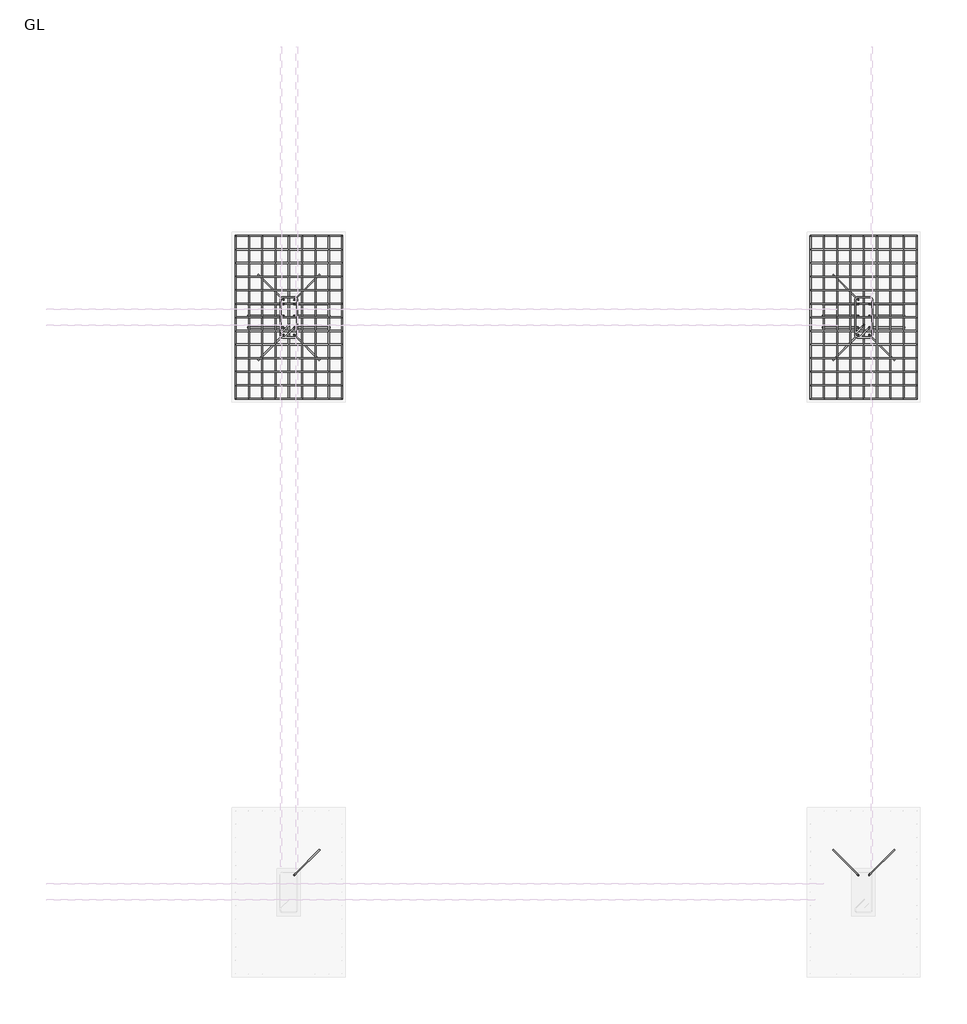
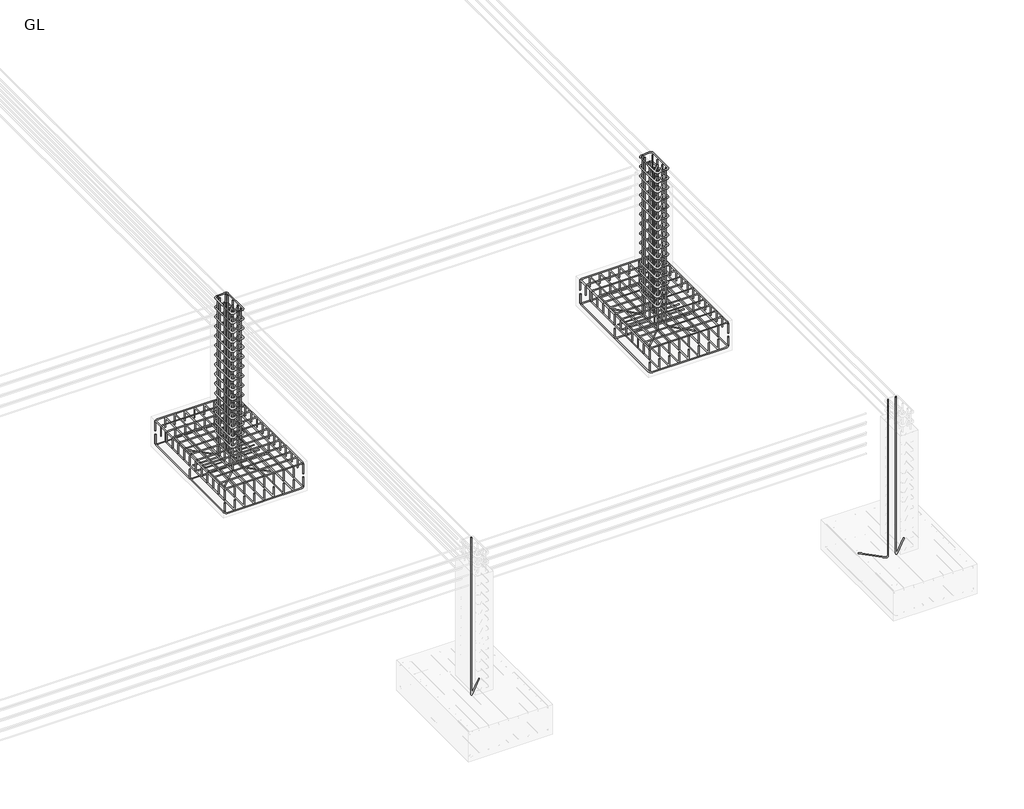
# One storey, part 11 of 16: 24 reinforcing bars.
"""IFC4 building model written with IfcOpenShell, lengths in millimetres."""

from ifc_helpers import new_model, si_unit, point, frame, origin, place, context, project, spatial, polyline, circle_curve, trimmed, segment, composite_curve, source, transform, mapped, element, save
from ifc_brep_helpers import swept_disk

model = new_model("IFC4")

# Units and contexts
model_context = context("Model", 3, world=origin())
ifc_project = project(units=[si_unit("LENGTHUNIT", "METRE", prefix="MILLI")], contexts=[model_context])

# Site, building, storey
site = spatial("IfcSite", under=ifc_project)
building = spatial("IfcBuilding", under=site)
storey = spatial("IfcBuildingStorey", under=building, Name="GL", Elevation=-1829.0)

# Reinforcing bars
placement = place(None, origin())
reinforcing_bar_shape = source(origin(), model_context, "Body", "SolidModel", [
    swept_disk(composite_curve([segment(polyline([(8237.0455621, -13319.1167521, -2089.0), (8237.0455621, -13319.1167521, -2213.0)]), True, "CONTINUOUS"), segment(trimmed(circle_curve(frame((8207.0455621, -13319.1167521, -2213.0), z_axis=(0.0, 1.0, 0.0), x_axis=(30.0, 0.0, 0.0)), 30.0), [point((8237.0455621, -13319.1167521, -2213.0))], [point((8207.0455621, -13319.1167521, -2243.0))], True, "CARTESIAN"), True, "CONTINUOUS"), segment(polyline([(8207.0455621, -13319.1167521, -2243.0), (7139.0455621, -13319.1167521, -2243.0)]), True, "CONTINUOUS"), segment(trimmed(circle_curve(frame((7139.0455621, -13319.1167521, -2213.0), z_axis=(0.0, 1.0, 0.0), x_axis=(0.0, 0.0, -30.0)), 30.0), [point((7139.0455621, -13319.1167521, -2243.0))], [point((7109.0455621, -13319.1167521, -2213.0))], True, "CARTESIAN"), True, "CONTINUOUS"), segment(polyline([(7109.0455621, -13319.1167521, -2213.0), (7109.0455621, -13319.1167521, -2089.0)]), True, "CONTINUOUS")], self_intersect=False), 6.0),
])
element("IfcReinforcingBar", 1, at=placement, inside=storey, context=model_context, shape_type="MappedRepresentation", body=[
    mapped(reinforcing_bar_shape, transform((0.0, 0.0, 0.0), x_axis=(1.0, 0.0, 0.0), y_axis=(0.0, 1.0, 0.0), z_axis=(0.0, 0.0, 1.0))),
    mapped(reinforcing_bar_shape, transform((0.0, -864.0, 0.0), x_axis=(1.0, 0.0, 0.0), y_axis=(0.0, 1.0, 0.0), z_axis=(0.0, 0.0, 1.0))),
    mapped(reinforcing_bar_shape, transform((0.0, -1728.0, 0.0), x_axis=(1.0, 0.0, 0.0), y_axis=(0.0, 1.0, 0.0), z_axis=(0.0, 0.0, 1.0))),
])
reinforcing_bar_2_shape = source(origin(), model_context, "Body", "SolidModel", [
    swept_disk(composite_curve([segment(polyline([(7109.0455621, -13319.1167521, -2022.436678), (7109.0455621, -13319.1167521, -1898.436678)]), True, "CONTINUOUS"), segment(trimmed(circle_curve(frame((7139.0455621, -13319.1167521, -1898.436678), z_axis=(0.0, 1.0, 0.0), x_axis=(-30.0, 0.0, 0.0)), 30.0), [point((7109.0455621, -13319.1167521, -1898.436678))], [point((7139.0455621, -13319.1167521, -1868.436678))], True, "CARTESIAN"), True, "CONTINUOUS"), segment(polyline([(7139.0455621, -13319.1167521, -1868.436678), (8207.0455621, -13319.1167521, -1868.436678)]), True, "CONTINUOUS"), segment(trimmed(circle_curve(frame((8207.0455621, -13319.1167521, -1898.436678), z_axis=(0.0, 1.0, 0.0), x_axis=(0.0, 0.0, 30.0)), 30.0), [point((8207.0455621, -13319.1167521, -1868.436678))], [point((8237.0455621, -13319.1167521, -1898.436678))], True, "CARTESIAN"), True, "CONTINUOUS"), segment(polyline([(8237.0455621, -13319.1167521, -1898.436678), (8237.0455621, -13319.1167521, -2022.436678)]), True, "CONTINUOUS")], self_intersect=False), 6.0),
])
element("IfcReinforcingBar", 2, at=placement, inside=storey, context=model_context, shape_type="MappedRepresentation", body=[
    mapped(reinforcing_bar_2_shape, transform((0.0, 0.0, 0.0), x_axis=(1.0, 0.0, 0.0), y_axis=(0.0, 1.0, 0.0), z_axis=(0.0, 0.0, 1.0))),
    mapped(reinforcing_bar_2_shape, transform((0.0, -144.0, 0.0), x_axis=(1.0, 0.0, 0.0), y_axis=(0.0, 1.0, 0.0), z_axis=(0.0, 0.0, 1.0))),
    mapped(reinforcing_bar_2_shape, transform((0.0, -288.0, 0.0), x_axis=(1.0, 0.0, 0.0), y_axis=(0.0, 1.0, 0.0), z_axis=(0.0, 0.0, 1.0))),
    mapped(reinforcing_bar_2_shape, transform((0.0, -432.0, 0.0), x_axis=(1.0, 0.0, 0.0), y_axis=(0.0, 1.0, 0.0), z_axis=(0.0, 0.0, 1.0))),
    mapped(reinforcing_bar_2_shape, transform((0.0, -576.0, 0.0), x_axis=(1.0, 0.0, 0.0), y_axis=(0.0, 1.0, 0.0), z_axis=(0.0, 0.0, 1.0))),
    mapped(reinforcing_bar_2_shape, transform((0.0, -720.0, 0.0), x_axis=(1.0, 0.0, 0.0), y_axis=(0.0, 1.0, 0.0), z_axis=(0.0, 0.0, 1.0))),
    mapped(reinforcing_bar_2_shape, transform((0.0, -864.0, 0.0), x_axis=(1.0, 0.0, 0.0), y_axis=(0.0, 1.0, 0.0), z_axis=(0.0, 0.0, 1.0))),
    mapped(reinforcing_bar_2_shape, transform((0.0, -1008.0, 0.0), x_axis=(1.0, 0.0, 0.0), y_axis=(0.0, 1.0, 0.0), z_axis=(0.0, 0.0, 1.0))),
    mapped(reinforcing_bar_2_shape, transform((0.0, -1152.0, 0.0), x_axis=(1.0, 0.0, 0.0), y_axis=(0.0, 1.0, 0.0), z_axis=(0.0, 0.0, 1.0))),
    mapped(reinforcing_bar_2_shape, transform((0.0, -1296.0, 0.0), x_axis=(1.0, 0.0, 0.0), y_axis=(0.0, 1.0, 0.0), z_axis=(0.0, 0.0, 1.0))),
    mapped(reinforcing_bar_2_shape, transform((0.0, -1440.0, 0.0), x_axis=(1.0, 0.0, 0.0), y_axis=(0.0, 1.0, 0.0), z_axis=(0.0, 0.0, 1.0))),
    mapped(reinforcing_bar_2_shape, transform((0.0, -1584.0, 0.0), x_axis=(1.0, 0.0, 0.0), y_axis=(0.0, 1.0, 0.0), z_axis=(0.0, 0.0, 1.0))),
    mapped(reinforcing_bar_2_shape, transform((0.0, -1728.0, 0.0), x_axis=(1.0, 0.0, 0.0), y_axis=(0.0, 1.0, 0.0), z_axis=(0.0, 0.0, 1.0))),
])
reinforcing_bar_3_shape = source(origin(), model_context, "Body", "SolidModel", [
    swept_disk(composite_curve([segment(polyline([(7109.0455621, -15047.1167521, -2027.5081232), (7109.0455621, -15047.1167521, -1903.5081232)]), True, "CONTINUOUS"), segment(trimmed(circle_curve(frame((7109.0455621, -15017.1167521, -1903.5081232), z_axis=(-1.0, 0.0, 0.0), x_axis=(0.0, -30.0, 0.0)), 30.0), [point((7109.0455621, -15047.1167521, -1903.5081232))], [point((7109.0455621, -15017.1167521, -1873.5081232))], True, "CARTESIAN"), True, "CONTINUOUS"), segment(polyline([(7109.0455621, -15017.1167521, -1873.5081232), (7109.0455621, -13349.1167521, -1873.5081232)]), True, "CONTINUOUS"), segment(trimmed(circle_curve(frame((7109.0455621, -13349.1167521, -1903.5081232), z_axis=(-1.0, 0.0, 0.0), x_axis=(0.0, 0.0, 30.0)), 30.0), [point((7109.0455621, -13349.1167521, -1873.5081232))], [point((7109.0455621, -13319.1167521, -1903.5081232))], True, "CARTESIAN"), True, "CONTINUOUS"), segment(polyline([(7109.0455621, -13319.1167521, -1903.5081232), (7109.0455621, -13319.1167521, -2027.5081232)]), True, "CONTINUOUS")], self_intersect=False), 6.0),
])
element("IfcReinforcingBar", 3, at=placement, inside=storey, context=model_context, shape_type="MappedRepresentation", body=[
    mapped(reinforcing_bar_3_shape, transform((0.0, 0.0, 0.0), x_axis=(1.0, 0.0, 0.0), y_axis=(0.0, 1.0, 0.0), z_axis=(0.0, 0.0, 1.0))),
    mapped(reinforcing_bar_3_shape, transform((141.0, 0.0, 0.0), x_axis=(1.0, 0.0, 0.0), y_axis=(0.0, 1.0, 0.0), z_axis=(0.0, 0.0, 1.0))),
    mapped(reinforcing_bar_3_shape, transform((282.0, 0.0, 0.0), x_axis=(1.0, 0.0, 0.0), y_axis=(0.0, 1.0, 0.0), z_axis=(0.0, 0.0, 1.0))),
    mapped(reinforcing_bar_3_shape, transform((423.0, 0.0, 0.0), x_axis=(1.0, 0.0, 0.0), y_axis=(0.0, 1.0, 0.0), z_axis=(0.0, 0.0, 1.0))),
    mapped(reinforcing_bar_3_shape, transform((564.0, 0.0, 0.0), x_axis=(1.0, 0.0, 0.0), y_axis=(0.0, 1.0, 0.0), z_axis=(0.0, 0.0, 1.0))),
    mapped(reinforcing_bar_3_shape, transform((705.0, 0.0, 0.0), x_axis=(1.0, 0.0, 0.0), y_axis=(0.0, 1.0, 0.0), z_axis=(0.0, 0.0, 1.0))),
    mapped(reinforcing_bar_3_shape, transform((846.0, 0.0, 0.0), x_axis=(1.0, 0.0, 0.0), y_axis=(0.0, 1.0, 0.0), z_axis=(0.0, 0.0, 1.0))),
    mapped(reinforcing_bar_3_shape, transform((987.0, 0.0, 0.0), x_axis=(1.0, 0.0, 0.0), y_axis=(0.0, 1.0, 0.0), z_axis=(0.0, 0.0, 1.0))),
    mapped(reinforcing_bar_3_shape, transform((1128.0, 0.0, 0.0), x_axis=(1.0, 0.0, 0.0), y_axis=(0.0, 1.0, 0.0), z_axis=(0.0, 0.0, 1.0))),
])
reinforcing_bar_4_shape = source(origin(), model_context, "Body", "SolidModel", [
    swept_disk(composite_curve([segment(polyline([(8237.0455621, -15047.1167521, -2080.6239909), (8237.0455621, -15047.1167521, -2204.6239909)]), True, "CONTINUOUS"), segment(trimmed(circle_curve(frame((8237.0455621, -15017.1167521, -2204.6239909), z_axis=(1.0, 0.0, 0.0), x_axis=(0.0, -30.0, 0.0)), 30.0), [point((8237.0455621, -15047.1167521, -2204.6239909))], [point((8237.0455621, -15017.1167521, -2234.6239909))], True, "CARTESIAN"), True, "CONTINUOUS"), segment(polyline([(8237.0455621, -15017.1167521, -2234.6239909), (8237.0455621, -13362.1421892, -2234.6239909)]), True, "CONTINUOUS"), segment(trimmed(circle_curve(frame((8237.0455621, -13362.1421892, -2204.6239909), z_axis=(1.0, 0.0, 0.0), x_axis=(0.0, 0.0, -30.0)), 30.0), [point((8237.0455621, -13362.1421892, -2234.6239909))], [point((8237.0455621, -13332.1421892, -2204.6239909))], True, "CARTESIAN"), True, "CONTINUOUS"), segment(polyline([(8237.0455621, -13332.1421892, -2204.6239909), (8237.0455621, -13332.1421892, -2080.6239909)]), True, "CONTINUOUS")], self_intersect=False), 6.0),
])
element("IfcReinforcingBar", 4, at=placement, inside=storey, context=model_context, shape_type="MappedRepresentation", body=[
    mapped(reinforcing_bar_4_shape, transform((0.0, 0.0, 0.0), x_axis=(1.0, 0.0, 0.0), y_axis=(0.0, 1.0, 0.0), z_axis=(0.0, 0.0, 1.0))),
    mapped(reinforcing_bar_4_shape, transform((-141.0, 0.0, 0.0), x_axis=(1.0, 0.0, 0.0), y_axis=(0.0, 1.0, 0.0), z_axis=(0.0, 0.0, 1.0))),
    mapped(reinforcing_bar_4_shape, transform((-282.0, 0.0, 0.0), x_axis=(1.0, 0.0, 0.0), y_axis=(0.0, 1.0, 0.0), z_axis=(0.0, 0.0, 1.0))),
    mapped(reinforcing_bar_4_shape, transform((-423.0, 0.0, 0.0), x_axis=(1.0, 0.0, 0.0), y_axis=(0.0, 1.0, 0.0), z_axis=(0.0, 0.0, 1.0))),
    mapped(reinforcing_bar_4_shape, transform((-564.0, 0.0, 0.0), x_axis=(1.0, 0.0, 0.0), y_axis=(0.0, 1.0, 0.0), z_axis=(0.0, 0.0, 1.0))),
    mapped(reinforcing_bar_4_shape, transform((-705.0, 0.0, 0.0), x_axis=(1.0, 0.0, 0.0), y_axis=(0.0, 1.0, 0.0), z_axis=(0.0, 0.0, 1.0))),
    mapped(reinforcing_bar_4_shape, transform((-846.0, 0.0, 0.0), x_axis=(1.0, 0.0, 0.0), y_axis=(0.0, 1.0, 0.0), z_axis=(0.0, 0.0, 1.0))),
    mapped(reinforcing_bar_4_shape, transform((-987.0, 0.0, 0.0), x_axis=(1.0, 0.0, 0.0), y_axis=(0.0, 1.0, 0.0), z_axis=(0.0, 0.0, 1.0))),
    mapped(reinforcing_bar_4_shape, transform((-1128.0, 0.0, 0.0), x_axis=(1.0, 0.0, 0.0), y_axis=(0.0, 1.0, 0.0), z_axis=(0.0, 0.0, 1.0))),
])
reinforcing_bar_5_shape = source(origin(), model_context, "Body", "SolidModel", [
    swept_disk(composite_curve([segment(polyline([(2141.0455621, -13319.1167521, -2089.0), (2141.0455621, -13319.1167521, -2213.0)]), True, "CONTINUOUS"), segment(trimmed(circle_curve(frame((2111.0455621, -13319.1167521, -2213.0), z_axis=(0.0, 1.0, 0.0), x_axis=(30.0, 0.0, 0.0)), 30.0), [point((2141.0455621, -13319.1167521, -2213.0))], [point((2111.0455621, -13319.1167521, -2243.0))], True, "CARTESIAN"), True, "CONTINUOUS"), segment(polyline([(2111.0455621, -13319.1167521, -2243.0), (1043.0455621, -13319.1167521, -2243.0)]), True, "CONTINUOUS"), segment(trimmed(circle_curve(frame((1043.0455621, -13319.1167521, -2213.0), z_axis=(0.0, 1.0, 0.0), x_axis=(0.0, 0.0, -30.0)), 30.0), [point((1043.0455621, -13319.1167521, -2243.0))], [point((1013.0455621, -13319.1167521, -2213.0))], True, "CARTESIAN"), True, "CONTINUOUS"), segment(polyline([(1013.0455621, -13319.1167521, -2213.0), (1013.0455621, -13319.1167521, -2089.0)]), True, "CONTINUOUS")], self_intersect=False), 6.0),
])
element("IfcReinforcingBar", 5, at=placement, inside=storey, context=model_context, shape_type="MappedRepresentation", body=[
    mapped(reinforcing_bar_5_shape, transform((0.0, 0.0, 0.0), x_axis=(1.0, 0.0, 0.0), y_axis=(0.0, 1.0, 0.0), z_axis=(0.0, 0.0, 1.0))),
    mapped(reinforcing_bar_5_shape, transform((0.0, -864.0, 0.0), x_axis=(1.0, 0.0, 0.0), y_axis=(0.0, 1.0, 0.0), z_axis=(0.0, 0.0, 1.0))),
    mapped(reinforcing_bar_5_shape, transform((0.0, -1728.0, 0.0), x_axis=(1.0, 0.0, 0.0), y_axis=(0.0, 1.0, 0.0), z_axis=(0.0, 0.0, 1.0))),
])
reinforcing_bar_6_shape = source(origin(), model_context, "Body", "SolidModel", [
    swept_disk(composite_curve([segment(polyline([(1013.0455621, -13319.1167521, -2022.436678), (1013.0455621, -13319.1167521, -1898.436678)]), True, "CONTINUOUS"), segment(trimmed(circle_curve(frame((1043.0455621, -13319.1167521, -1898.436678), z_axis=(0.0, 1.0, 0.0), x_axis=(-30.000000000000114, 0.0, 0.0)), 30.0), [point((1013.0455621, -13319.1167521, -1898.436678))], [point((1043.0455621, -13319.1167521, -1868.436678))], True, "CARTESIAN"), True, "CONTINUOUS"), segment(polyline([(1043.0455621, -13319.1167521, -1868.436678), (2111.0455621, -13319.1167521, -1868.436678)]), True, "CONTINUOUS"), segment(trimmed(circle_curve(frame((2111.0455621, -13319.1167521, -1898.436678), z_axis=(0.0, 1.0, 0.0), x_axis=(0.0, 0.0, 30.0)), 30.0), [point((2111.0455621, -13319.1167521, -1868.436678))], [point((2141.0455621, -13319.1167521, -1898.436678))], True, "CARTESIAN"), True, "CONTINUOUS"), segment(polyline([(2141.0455621, -13319.1167521, -1898.436678), (2141.0455621, -13319.1167521, -2022.436678)]), True, "CONTINUOUS")], self_intersect=False), 6.0),
])
element("IfcReinforcingBar", 6, at=placement, inside=storey, context=model_context, shape_type="MappedRepresentation", body=[
    mapped(reinforcing_bar_6_shape, transform((0.0, 0.0, 0.0), x_axis=(1.0, 0.0, 0.0), y_axis=(0.0, 1.0, 0.0), z_axis=(0.0, 0.0, 1.0))),
    mapped(reinforcing_bar_6_shape, transform((0.0, -144.0, 0.0), x_axis=(1.0, 0.0, 0.0), y_axis=(0.0, 1.0, 0.0), z_axis=(0.0, 0.0, 1.0))),
    mapped(reinforcing_bar_6_shape, transform((0.0, -288.0, 0.0), x_axis=(1.0, 0.0, 0.0), y_axis=(0.0, 1.0, 0.0), z_axis=(0.0, 0.0, 1.0))),
    mapped(reinforcing_bar_6_shape, transform((0.0, -432.0, 0.0), x_axis=(1.0, 0.0, 0.0), y_axis=(0.0, 1.0, 0.0), z_axis=(0.0, 0.0, 1.0))),
    mapped(reinforcing_bar_6_shape, transform((0.0, -576.0, 0.0), x_axis=(1.0, 0.0, 0.0), y_axis=(0.0, 1.0, 0.0), z_axis=(0.0, 0.0, 1.0))),
    mapped(reinforcing_bar_6_shape, transform((0.0, -720.0, 0.0), x_axis=(1.0, 0.0, 0.0), y_axis=(0.0, 1.0, 0.0), z_axis=(0.0, 0.0, 1.0))),
    mapped(reinforcing_bar_6_shape, transform((0.0, -864.0, 0.0), x_axis=(1.0, 0.0, 0.0), y_axis=(0.0, 1.0, 0.0), z_axis=(0.0, 0.0, 1.0))),
    mapped(reinforcing_bar_6_shape, transform((0.0, -1008.0, 0.0), x_axis=(1.0, 0.0, 0.0), y_axis=(0.0, 1.0, 0.0), z_axis=(0.0, 0.0, 1.0))),
    mapped(reinforcing_bar_6_shape, transform((0.0, -1152.0, 0.0), x_axis=(1.0, 0.0, 0.0), y_axis=(0.0, 1.0, 0.0), z_axis=(0.0, 0.0, 1.0))),
    mapped(reinforcing_bar_6_shape, transform((0.0, -1296.0, 0.0), x_axis=(1.0, 0.0, 0.0), y_axis=(0.0, 1.0, 0.0), z_axis=(0.0, 0.0, 1.0))),
    mapped(reinforcing_bar_6_shape, transform((0.0, -1440.0, 0.0), x_axis=(1.0, 0.0, 0.0), y_axis=(0.0, 1.0, 0.0), z_axis=(0.0, 0.0, 1.0))),
    mapped(reinforcing_bar_6_shape, transform((0.0, -1584.0, 0.0), x_axis=(1.0, 0.0, 0.0), y_axis=(0.0, 1.0, 0.0), z_axis=(0.0, 0.0, 1.0))),
    mapped(reinforcing_bar_6_shape, transform((0.0, -1728.0, 0.0), x_axis=(1.0, 0.0, 0.0), y_axis=(0.0, 1.0, 0.0), z_axis=(0.0, 0.0, 1.0))),
])
reinforcing_bar_7_shape = source(origin(), model_context, "Body", "SolidModel", [
    swept_disk(composite_curve([segment(polyline([(1013.0455621, -15047.1167521, -2027.5081232), (1013.0455621, -15047.1167521, -1903.5081232)]), True, "CONTINUOUS"), segment(trimmed(circle_curve(frame((1013.0455621, -15017.1167521, -1903.5081232), z_axis=(-1.0, 0.0, 0.0), x_axis=(0.0, -30.0, 0.0)), 30.0), [point((1013.0455621, -15047.1167521, -1903.5081232))], [point((1013.0455621, -15017.1167521, -1873.5081232))], True, "CARTESIAN"), True, "CONTINUOUS"), segment(polyline([(1013.0455621, -15017.1167521, -1873.5081232), (1013.0455621, -13349.1167521, -1873.5081232)]), True, "CONTINUOUS"), segment(trimmed(circle_curve(frame((1013.0455621, -13349.1167521, -1903.5081232), z_axis=(-1.0, 0.0, 0.0), x_axis=(0.0, 0.0, 30.0)), 30.0), [point((1013.0455621, -13349.1167521, -1873.5081232))], [point((1013.0455621, -13319.1167521, -1903.5081232))], True, "CARTESIAN"), True, "CONTINUOUS"), segment(polyline([(1013.0455621, -13319.1167521, -1903.5081232), (1013.0455621, -13319.1167521, -2027.5081232)]), True, "CONTINUOUS")], self_intersect=False), 6.0),
])
element("IfcReinforcingBar", 7, at=placement, inside=storey, context=model_context, shape_type="MappedRepresentation", body=[
    mapped(reinforcing_bar_7_shape, transform((0.0, 0.0, 0.0), x_axis=(1.0, 0.0, 0.0), y_axis=(0.0, 1.0, 0.0), z_axis=(0.0, 0.0, 1.0))),
    mapped(reinforcing_bar_7_shape, transform((141.0, 0.0, 0.0), x_axis=(1.0, 0.0, 0.0), y_axis=(0.0, 1.0, 0.0), z_axis=(0.0, 0.0, 1.0))),
    mapped(reinforcing_bar_7_shape, transform((282.0, 0.0, 0.0), x_axis=(1.0, 0.0, 0.0), y_axis=(0.0, 1.0, 0.0), z_axis=(0.0, 0.0, 1.0))),
    mapped(reinforcing_bar_7_shape, transform((423.0, 0.0, 0.0), x_axis=(1.0, 0.0, 0.0), y_axis=(0.0, 1.0, 0.0), z_axis=(0.0, 0.0, 1.0))),
    mapped(reinforcing_bar_7_shape, transform((564.0, 0.0, 0.0), x_axis=(1.0, 0.0, 0.0), y_axis=(0.0, 1.0, 0.0), z_axis=(0.0, 0.0, 1.0))),
    mapped(reinforcing_bar_7_shape, transform((705.0, 0.0, 0.0), x_axis=(1.0, 0.0, 0.0), y_axis=(0.0, 1.0, 0.0), z_axis=(0.0, 0.0, 1.0))),
    mapped(reinforcing_bar_7_shape, transform((846.0, 0.0, 0.0), x_axis=(1.0, 0.0, 0.0), y_axis=(0.0, 1.0, 0.0), z_axis=(0.0, 0.0, 1.0))),
    mapped(reinforcing_bar_7_shape, transform((987.0, 0.0, 0.0), x_axis=(1.0, 0.0, 0.0), y_axis=(0.0, 1.0, 0.0), z_axis=(0.0, 0.0, 1.0))),
    mapped(reinforcing_bar_7_shape, transform((1128.0, 0.0, 0.0), x_axis=(1.0, 0.0, 0.0), y_axis=(0.0, 1.0, 0.0), z_axis=(0.0, 0.0, 1.0))),
])
reinforcing_bar_8_shape = source(origin(), model_context, "Body", "SolidModel", [
    swept_disk(composite_curve([segment(polyline([(2141.0455621, -15047.1167521, -2080.6239909), (2141.0455621, -15047.1167521, -2204.6239909)]), True, "CONTINUOUS"), segment(trimmed(circle_curve(frame((2141.0455621, -15017.1167521, -2204.6239909), z_axis=(1.0, 0.0, 0.0), x_axis=(0.0, -30.0, 0.0)), 30.0), [point((2141.0455621, -15047.1167521, -2204.6239909))], [point((2141.0455621, -15017.1167521, -2234.6239909))], True, "CARTESIAN"), True, "CONTINUOUS"), segment(polyline([(2141.0455621, -15017.1167521, -2234.6239909), (2141.0455621, -13362.1421892, -2234.6239909)]), True, "CONTINUOUS"), segment(trimmed(circle_curve(frame((2141.0455621, -13362.1421892, -2204.6239909), z_axis=(1.0, 0.0, 0.0), x_axis=(0.0, 0.0, -30.0)), 30.0), [point((2141.0455621, -13362.1421892, -2234.6239909))], [point((2141.0455621, -13332.1421892, -2204.6239909))], True, "CARTESIAN"), True, "CONTINUOUS"), segment(polyline([(2141.0455621, -13332.1421892, -2204.6239909), (2141.0455621, -13332.1421892, -2080.6239909)]), True, "CONTINUOUS")], self_intersect=False), 6.0),
])
element("IfcReinforcingBar", 8, at=placement, inside=storey, context=model_context, shape_type="MappedRepresentation", body=[
    mapped(reinforcing_bar_8_shape, transform((0.0, 0.0, 0.0), x_axis=(1.0, 0.0, 0.0), y_axis=(0.0, 1.0, 0.0), z_axis=(0.0, 0.0, 1.0))),
    mapped(reinforcing_bar_8_shape, transform((-141.0, 0.0, 0.0), x_axis=(1.0, 0.0, 0.0), y_axis=(0.0, 1.0, 0.0), z_axis=(0.0, 0.0, 1.0))),
    mapped(reinforcing_bar_8_shape, transform((-282.0, 0.0, 0.0), x_axis=(1.0, 0.0, 0.0), y_axis=(0.0, 1.0, 0.0), z_axis=(0.0, 0.0, 1.0))),
    mapped(reinforcing_bar_8_shape, transform((-423.0, 0.0, 0.0), x_axis=(1.0, 0.0, 0.0), y_axis=(0.0, 1.0, 0.0), z_axis=(0.0, 0.0, 1.0))),
    mapped(reinforcing_bar_8_shape, transform((-564.0, 0.0, 0.0), x_axis=(1.0, 0.0, 0.0), y_axis=(0.0, 1.0, 0.0), z_axis=(0.0, 0.0, 1.0))),
    mapped(reinforcing_bar_8_shape, transform((-705.0, 0.0, 0.0), x_axis=(1.0, 0.0, 0.0), y_axis=(0.0, 1.0, 0.0), z_axis=(0.0, 0.0, 1.0))),
    mapped(reinforcing_bar_8_shape, transform((-846.0, 0.0, 0.0), x_axis=(1.0, 0.0, 0.0), y_axis=(0.0, 1.0, 0.0), z_axis=(0.0, 0.0, 1.0))),
    mapped(reinforcing_bar_8_shape, transform((-987.0, 0.0, 0.0), x_axis=(1.0, 0.0, 0.0), y_axis=(0.0, 1.0, 0.0), z_axis=(0.0, 0.0, 1.0))),
    mapped(reinforcing_bar_8_shape, transform((-1128.0, 0.0, 0.0), x_axis=(1.0, 0.0, 0.0), y_axis=(0.0, 1.0, 0.0), z_axis=(0.0, 0.0, 1.0))),
])
element("IfcReinforcingBar", 9, at=placement, inside=storey, context=model_context, shape_type="SolidModel", body=[
    swept_disk(composite_curve([segment(polyline([(7615.9357768, -20094.1692603, 241.0), (7615.9357768, -20094.1692603, -2129.0)]), True, "CONTINUOUS"), segment(trimmed(circle_curve(frame((7594.7225734, -20072.9560568, -2129.0), z_axis=(0.7071067811865218, 0.7071067811865733, 0.0), x_axis=(21.213203399999657, -21.21320349999951, 0.0)), 30.0), [point((7615.9357768, -20094.1692603, -2129.0))], [point((7594.7225734, -20072.9560568, -2159.0))], True, "CARTESIAN"), True, "CONTINUOUS"), segment(polyline([(7594.7225734, -20072.9560568, -2159.0), (7347.2352, -19825.4686834, -2159.0)]), True, "CONTINUOUS")], self_intersect=False), 6.0),
])
element("IfcReinforcingBar", 10, at=placement, inside=storey, context=model_context, shape_type="SolidModel", body=[
    swept_disk(composite_curve([segment(polyline([(7730.1553473, -20094.1692603, 241.0), (7730.1553473, -20094.1692603, -2129.0)]), True, "CONTINUOUS"), segment(trimmed(circle_curve(frame((7751.3685508, -20072.9560568, -2129.0), z_axis=(0.7071067811865157, -0.7071067811865794, 0.0), x_axis=(-21.21320349999951, -21.21320349999951, 0.0)), 30.0), [point((7730.1553473, -20094.1692603, -2129.0))], [point((7751.3685508, -20072.9560568, -2159.0))], True, "CARTESIAN"), True, "CONTINUOUS"), segment(polyline([(7751.3685508, -20072.9560568, -2159.0), (7998.8559242, -19825.4686834, -2159.0)]), True, "CONTINUOUS")], self_intersect=False), 6.0),
])
reinforcing_bar_9_shape = source(origin(), model_context, "Body", "SolidModel", [
    swept_disk(composite_curve([segment(polyline([(7680.5135995, -14258.2223078, -1793.0), (7592.8323586, -14345.9035486, -1793.0)]), True, "CONTINUOUS"), segment(trimmed(circle_curve(frame((7614.0455621, -14367.1167521, -1793.0), z_axis=(0.0, 0.0, 1.0), x_axis=(-21.213203500000418, 21.213203500001327, 0.0)), 30.0), [point((7592.8323586, -14345.9035486, -1793.0))], [point((7614.0455621, -14397.1167521, -1793.0))], True, "CARTESIAN"), True, "CONTINUOUS"), segment(polyline([(7614.0455621, -14397.1167521, -1793.0), (7732.0455621, -14397.1167521, -1793.0)]), True, "CONTINUOUS"), segment(trimmed(circle_curve(frame((7732.0455621, -14367.1167521, -1793.0), z_axis=(0.0, 0.0, 1.0), x_axis=(0.0, -30.0, 0.0)), 30.0), [point((7732.0455621, -14397.1167521, -1793.0))], [point((7762.0455621, -14367.1167521, -1793.0))], True, "CARTESIAN"), True, "CONTINUOUS"), segment(polyline([(7762.0455621, -14367.1167521, -1793.0), (7762.0455621, -13999.1167521, -1793.0)]), True, "CONTINUOUS"), segment(trimmed(circle_curve(frame((7732.1135038, -13999.1167521, -1795.0178916), z_axis=(-0.06726305234213417, 0.0, 0.9977352764083365), x_axis=(29.93205829999988, 0.0, 2.0178915999999845)), 30.0), [point((7762.0455621, -13999.1167521, -1793.0))], [point((7732.1135038, -13969.1167521, -1795.0178916))], True, "CARTESIAN"), True, "CONTINUOUS"), segment(polyline([(7732.1135038, -13969.1167521, -1795.0178916), (7613.9776204, -13969.1167521, -1802.9821084)]), True, "CONTINUOUS"), segment(trimmed(circle_curve(frame((7613.9776204, -13999.1167521, -1802.9821084), z_axis=(-0.06726305234213417, 0.0, 0.9977352764083365), x_axis=(0.0, 30.0, 0.0)), 30.0), [point((7613.9776204, -13969.1167521, -1802.9821084))], [point((7584.0455621, -13999.1167521, -1805.0))], True, "CARTESIAN"), True, "CONTINUOUS"), segment(polyline([(7584.0455621, -13999.1167521, -1805.0), (7584.0455621, -14367.1167521, -1805.0)]), True, "CONTINUOUS"), segment(trimmed(circle_curve(frame((7614.0455621, -14367.1167521, -1805.0), z_axis=(0.0, 0.0, 1.0), x_axis=(-30.0, 0.0, 0.0)), 30.0), [point((7584.0455621, -14367.1167521, -1805.0))], [point((7635.2587655, -14388.3299555, -1805.0))], True, "CARTESIAN"), True, "CONTINUOUS"), segment(polyline([(7635.2587655, -14388.3299555, -1805.0), (7722.9400064, -14300.6487146, -1805.0)]), True, "CONTINUOUS")], self_intersect=False), 6.0),
])
element("IfcReinforcingBar", 11, at=placement, inside=storey, context=model_context, shape_type="MappedRepresentation", body=[
    mapped(reinforcing_bar_9_shape, transform((0.0, 0.0, 0.0), x_axis=(1.0, 0.0, 0.0), y_axis=(0.0, 1.0, 0.0), z_axis=(0.0, 0.0, 1.0))),
    mapped(reinforcing_bar_9_shape, transform((0.0, 0.0, 144.8571429), x_axis=(1.0, 0.0, 0.0), y_axis=(0.0, 1.0, 0.0), z_axis=(0.0, 0.0, 1.0))),
    mapped(reinforcing_bar_9_shape, transform((0.0, 0.0, 289.7142857), x_axis=(1.0, 0.0, 0.0), y_axis=(0.0, 1.0, 0.0), z_axis=(0.0, 0.0, 1.0))),
    mapped(reinforcing_bar_9_shape, transform((0.0, 0.0, 434.5714286), x_axis=(1.0, 0.0, 0.0), y_axis=(0.0, 1.0, 0.0), z_axis=(0.0, 0.0, 1.0))),
    mapped(reinforcing_bar_9_shape, transform((0.0, 0.0, 579.4285714), x_axis=(1.0, 0.0, 0.0), y_axis=(0.0, 1.0, 0.0), z_axis=(0.0, 0.0, 1.0))),
    mapped(reinforcing_bar_9_shape, transform((0.0, 0.0, 724.2857143), x_axis=(1.0, 0.0, 0.0), y_axis=(0.0, 1.0, 0.0), z_axis=(0.0, 0.0, 1.0))),
    mapped(reinforcing_bar_9_shape, transform((0.0, 0.0, 869.1428571), x_axis=(1.0, 0.0, 0.0), y_axis=(0.0, 1.0, 0.0), z_axis=(0.0, 0.0, 1.0))),
    mapped(reinforcing_bar_9_shape, transform((0.0, 0.0, 1014.0), x_axis=(1.0, 0.0, 0.0), y_axis=(0.0, 1.0, 0.0), z_axis=(0.0, 0.0, 1.0))),
    mapped(reinforcing_bar_9_shape, transform((0.0, 0.0, 1158.8571429), x_axis=(1.0, 0.0, 0.0), y_axis=(0.0, 1.0, 0.0), z_axis=(0.0, 0.0, 1.0))),
    mapped(reinforcing_bar_9_shape, transform((0.0, 0.0, 1303.7142857), x_axis=(1.0, 0.0, 0.0), y_axis=(0.0, 1.0, 0.0), z_axis=(0.0, 0.0, 1.0))),
    mapped(reinforcing_bar_9_shape, transform((0.0, 0.0, 1448.5714286), x_axis=(1.0, 0.0, 0.0), y_axis=(0.0, 1.0, 0.0), z_axis=(0.0, 0.0, 1.0))),
    mapped(reinforcing_bar_9_shape, transform((0.0, 0.0, 1593.4285714), x_axis=(1.0, 0.0, 0.0), y_axis=(0.0, 1.0, 0.0), z_axis=(0.0, 0.0, 1.0))),
    mapped(reinforcing_bar_9_shape, transform((0.0, 0.0, 1738.2857143), x_axis=(1.0, 0.0, 0.0), y_axis=(0.0, 1.0, 0.0), z_axis=(0.0, 0.0, 1.0))),
    mapped(reinforcing_bar_9_shape, transform((0.0, 0.0, 1883.1428571), x_axis=(1.0, 0.0, 0.0), y_axis=(0.0, 1.0, 0.0), z_axis=(0.0, 0.0, 1.0))),
    mapped(reinforcing_bar_9_shape, transform((0.0, 0.0, 2028.0), x_axis=(1.0, 0.0, 0.0), y_axis=(0.0, 1.0, 0.0), z_axis=(0.0, 0.0, 1.0))),
])
element("IfcReinforcingBar", 12, at=placement, inside=storey, context=model_context, shape_type="SolidModel", body=[
    swept_disk(composite_curve([segment(polyline([(7615.9357768, -14368.0642439, 241.0), (7615.9357768, -14368.0642439, -2129.0)]), True, "CONTINUOUS"), segment(trimmed(circle_curve(frame((7594.7225734, -14389.2774473, -2129.0), z_axis=(-0.7071067811865187, 0.7071067811865764, 0.0), x_axis=(21.213203399999657, 21.213203400000566, 0.0)), 30.0), [point((7615.9357768, -14368.0642439, -2129.0))], [point((7594.7225734, -14389.2774473, -2159.0))], True, "CARTESIAN"), True, "CONTINUOUS"), segment(polyline([(7594.7225734, -14389.2774473, -2159.0), (7347.2352, -14636.7648207, -2159.0)]), True, "CONTINUOUS")], self_intersect=False), 6.0),
])
element("IfcReinforcingBar", 13, at=placement, inside=storey, context=model_context, shape_type="SolidModel", body=[
    swept_disk(composite_curve([segment(polyline([(7615.9357768, -13998.1692603, 241.0), (7615.9357768, -13998.1692603, -2129.0)]), True, "CONTINUOUS"), segment(trimmed(circle_curve(frame((7594.7225734, -13976.9560568, -2129.0), z_axis=(0.7071067811865218, 0.7071067811865733, 0.0), x_axis=(21.213203399999657, -21.21320349999951, 0.0)), 30.0), [point((7615.9357768, -13998.1692603, -2129.0))], [point((7594.7225734, -13976.9560568, -2159.0))], True, "CARTESIAN"), True, "CONTINUOUS"), segment(polyline([(7594.7225734, -13976.9560568, -2159.0), (7347.2352, -13729.4686834, -2159.0)]), True, "CONTINUOUS")], self_intersect=False), 6.0),
])
element("IfcReinforcingBar", 14, at=placement, inside=storey, context=model_context, shape_type="SolidModel", body=[
    swept_disk(composite_curve([segment(polyline([(7730.1553473, -14368.0642439, 241.0), (7730.1553473, -14368.0642439, -2129.0)]), True, "CONTINUOUS"), segment(trimmed(circle_curve(frame((7751.3685508, -14389.2774473, -2129.0), z_axis=(-0.7071067811865248, -0.7071067811865703, 0.0), x_axis=(-21.21320349999951, 21.213203400000566, 0.0)), 30.0), [point((7730.1553473, -14368.0642439, -2129.0))], [point((7751.3685508, -14389.2774473, -2159.0))], True, "CARTESIAN"), True, "CONTINUOUS"), segment(polyline([(7751.3685508, -14389.2774473, -2159.0), (7998.8559242, -14636.7648207, -2159.0)]), True, "CONTINUOUS")], self_intersect=False), 6.0),
])
reinforcing_bar_10_shape = source(origin(), model_context, "Body", "SolidModel", [
    swept_disk(composite_curve([segment(polyline([(7615.9357768, -14290.9117405, 241.0), (7615.9357768, -14290.9117405, -2129.0)]), True, "CONTINUOUS"), segment(trimmed(circle_curve(frame((7585.9357768, -14290.9117405, -2129.0), z_axis=(0.0, 1.0, 0.0), x_axis=(30.0, 0.0, 0.0)), 30.0), [point((7615.9357768, -14290.9117405, -2129.0))], [point((7585.9357768, -14290.9117405, -2159.0))], True, "CARTESIAN"), True, "CONTINUOUS"), segment(polyline([(7585.9357768, -14290.9117405, -2159.0), (7235.9357768, -14290.9117405, -2159.0)]), True, "CONTINUOUS")], self_intersect=False), 6.0),
])
element("IfcReinforcingBar", 15, at=placement, inside=storey, context=model_context, shape_type="MappedRepresentation", body=[
    mapped(reinforcing_bar_10_shape, transform((0.0, 0.0, 0.0), x_axis=(1.0, 0.0, 0.0), y_axis=(0.0, 1.0, 0.0), z_axis=(0.0, 0.0, 1.0))),
    mapped(reinforcing_bar_10_shape, transform((0.0, 123.5823926, 0.0), x_axis=(1.0, 0.0, 0.0), y_axis=(0.0, 1.0, 0.0), z_axis=(0.0, 0.0, 1.0))),
    mapped(reinforcing_bar_10_shape, transform((0.0, 247.1647853, 0.0), x_axis=(1.0, 0.0, 0.0), y_axis=(0.0, 1.0, 0.0), z_axis=(0.0, 0.0, 1.0))),
])
reinforcing_bar_11_shape = source(origin(), model_context, "Body", "SolidModel", [
    swept_disk(composite_curve([segment(polyline([(7730.1553473, -14290.9117405, 241.0), (7730.1553473, -14290.9117405, -2129.0)]), True, "CONTINUOUS"), segment(trimmed(circle_curve(frame((7760.1553473, -14290.9117405, -2129.0), z_axis=(0.0, -1.0, 0.0), x_axis=(-30.0, 0.0, 0.0)), 30.0), [point((7730.1553473, -14290.9117405, -2129.0))], [point((7760.1553473, -14290.9117405, -2159.0))], True, "CARTESIAN"), True, "CONTINUOUS"), segment(polyline([(7760.1553473, -14290.9117405, -2159.0), (8110.1553473, -14290.9117405, -2159.0)]), True, "CONTINUOUS")], self_intersect=False), 6.0),
])
element("IfcReinforcingBar", 16, at=placement, inside=storey, context=model_context, shape_type="MappedRepresentation", body=[
    mapped(reinforcing_bar_11_shape, transform((0.0, 0.0, 0.0), x_axis=(1.0, 0.0, 0.0), y_axis=(0.0, 1.0, 0.0), z_axis=(0.0, 0.0, 1.0))),
    mapped(reinforcing_bar_11_shape, transform((0.0, 123.5823926, 0.0), x_axis=(1.0, 0.0, 0.0), y_axis=(0.0, 1.0, 0.0), z_axis=(0.0, 0.0, 1.0))),
    mapped(reinforcing_bar_11_shape, transform((0.0, 247.1647853, 0.0), x_axis=(1.0, 0.0, 0.0), y_axis=(0.0, 1.0, 0.0), z_axis=(0.0, 0.0, 1.0))),
])
reinforcing_bar_12_shape = source(origin(), model_context, "Body", "SolidModel", [
    swept_disk(composite_curve([segment(polyline([(1584.5135995, -14258.2223078, -1793.0), (1496.8323586, -14345.9035486, -1793.0)]), True, "CONTINUOUS"), segment(trimmed(circle_curve(frame((1518.0455621, -14367.1167521, -1793.0), z_axis=(0.0, 0.0, 1.0), x_axis=(-21.21320350000019, 21.213203500001327, 0.0)), 30.0), [point((1496.8323586, -14345.9035486, -1793.0))], [point((1518.0455621, -14397.1167521, -1793.0))], True, "CARTESIAN"), True, "CONTINUOUS"), segment(polyline([(1518.0455621, -14397.1167521, -1793.0), (1636.0455621, -14397.1167521, -1793.0)]), True, "CONTINUOUS"), segment(trimmed(circle_curve(frame((1636.0455621, -14367.1167521, -1793.0), z_axis=(0.0, 0.0, 1.0), x_axis=(0.0, -30.0, 0.0)), 30.0), [point((1636.0455621, -14397.1167521, -1793.0))], [point((1666.0455621, -14367.1167521, -1793.0))], True, "CARTESIAN"), True, "CONTINUOUS"), segment(polyline([(1666.0455621, -14367.1167521, -1793.0), (1666.0455621, -13999.1167521, -1793.0)]), True, "CONTINUOUS"), segment(trimmed(circle_curve(frame((1636.1135038, -13999.1167521, -1795.0178916), z_axis=(-0.06726305234213417, 0.0, 0.9977352764083365), x_axis=(29.932058300000108, 0.0, 2.0178915999999845)), 30.0), [point((1666.0455621, -13999.1167521, -1793.0))], [point((1636.1135038, -13969.1167521, -1795.0178916))], True, "CARTESIAN"), True, "CONTINUOUS"), segment(polyline([(1636.1135038, -13969.1167521, -1795.0178916), (1517.9776204, -13969.1167521, -1802.9821084)]), True, "CONTINUOUS"), segment(trimmed(circle_curve(frame((1517.9776204, -13999.1167521, -1802.9821084), z_axis=(-0.06726305234213417, 0.0, 0.9977352764083365), x_axis=(0.0, 30.0, 0.0)), 30.0), [point((1517.9776204, -13969.1167521, -1802.9821084))], [point((1488.0455621, -13999.1167521, -1805.0))], True, "CARTESIAN"), True, "CONTINUOUS"), segment(polyline([(1488.0455621, -13999.1167521, -1805.0), (1488.0455621, -14367.1167521, -1805.0)]), True, "CONTINUOUS"), segment(trimmed(circle_curve(frame((1518.0455621, -14367.1167521, -1805.0), z_axis=(0.0, 0.0, 1.0), x_axis=(-30.0, 0.0, 0.0)), 30.0), [point((1488.0455621, -14367.1167521, -1805.0))], [point((1539.2587655, -14388.3299555, -1805.0))], True, "CARTESIAN"), True, "CONTINUOUS"), segment(polyline([(1539.2587655, -14388.3299555, -1805.0), (1626.9400064, -14300.6487146, -1805.0)]), True, "CONTINUOUS")], self_intersect=False), 6.0),
])
element("IfcReinforcingBar", 17, at=placement, inside=storey, context=model_context, shape_type="MappedRepresentation", body=[
    mapped(reinforcing_bar_12_shape, transform((0.0, 0.0, 0.0), x_axis=(1.0, 0.0, 0.0), y_axis=(0.0, 1.0, 0.0), z_axis=(0.0, 0.0, 1.0))),
    mapped(reinforcing_bar_12_shape, transform((0.0, 0.0, 144.8571429), x_axis=(1.0, 0.0, 0.0), y_axis=(0.0, 1.0, 0.0), z_axis=(0.0, 0.0, 1.0))),
    mapped(reinforcing_bar_12_shape, transform((0.0, 0.0, 289.7142857), x_axis=(1.0, 0.0, 0.0), y_axis=(0.0, 1.0, 0.0), z_axis=(0.0, 0.0, 1.0))),
    mapped(reinforcing_bar_12_shape, transform((0.0, 0.0, 434.5714286), x_axis=(1.0, 0.0, 0.0), y_axis=(0.0, 1.0, 0.0), z_axis=(0.0, 0.0, 1.0))),
    mapped(reinforcing_bar_12_shape, transform((0.0, 0.0, 579.4285714), x_axis=(1.0, 0.0, 0.0), y_axis=(0.0, 1.0, 0.0), z_axis=(0.0, 0.0, 1.0))),
    mapped(reinforcing_bar_12_shape, transform((0.0, 0.0, 724.2857143), x_axis=(1.0, 0.0, 0.0), y_axis=(0.0, 1.0, 0.0), z_axis=(0.0, 0.0, 1.0))),
    mapped(reinforcing_bar_12_shape, transform((0.0, 0.0, 869.1428571), x_axis=(1.0, 0.0, 0.0), y_axis=(0.0, 1.0, 0.0), z_axis=(0.0, 0.0, 1.0))),
    mapped(reinforcing_bar_12_shape, transform((0.0, 0.0, 1014.0), x_axis=(1.0, 0.0, 0.0), y_axis=(0.0, 1.0, 0.0), z_axis=(0.0, 0.0, 1.0))),
    mapped(reinforcing_bar_12_shape, transform((0.0, 0.0, 1158.8571429), x_axis=(1.0, 0.0, 0.0), y_axis=(0.0, 1.0, 0.0), z_axis=(0.0, 0.0, 1.0))),
    mapped(reinforcing_bar_12_shape, transform((0.0, 0.0, 1303.7142857), x_axis=(1.0, 0.0, 0.0), y_axis=(0.0, 1.0, 0.0), z_axis=(0.0, 0.0, 1.0))),
    mapped(reinforcing_bar_12_shape, transform((0.0, 0.0, 1448.5714286), x_axis=(1.0, 0.0, 0.0), y_axis=(0.0, 1.0, 0.0), z_axis=(0.0, 0.0, 1.0))),
    mapped(reinforcing_bar_12_shape, transform((0.0, 0.0, 1593.4285714), x_axis=(1.0, 0.0, 0.0), y_axis=(0.0, 1.0, 0.0), z_axis=(0.0, 0.0, 1.0))),
    mapped(reinforcing_bar_12_shape, transform((0.0, 0.0, 1738.2857143), x_axis=(1.0, 0.0, 0.0), y_axis=(0.0, 1.0, 0.0), z_axis=(0.0, 0.0, 1.0))),
    mapped(reinforcing_bar_12_shape, transform((0.0, 0.0, 1883.1428571), x_axis=(1.0, 0.0, 0.0), y_axis=(0.0, 1.0, 0.0), z_axis=(0.0, 0.0, 1.0))),
    mapped(reinforcing_bar_12_shape, transform((0.0, 0.0, 2028.0), x_axis=(1.0, 0.0, 0.0), y_axis=(0.0, 1.0, 0.0), z_axis=(0.0, 0.0, 1.0))),
])
element("IfcReinforcingBar", 18, at=placement, inside=storey, context=model_context, shape_type="SolidModel", body=[
    swept_disk(composite_curve([segment(polyline([(1519.9357768, -14368.0642439, 241.0), (1519.9357768, -14368.0642439, -2129.0)]), True, "CONTINUOUS"), segment(trimmed(circle_curve(frame((1498.7225734, -14389.2774473, -2129.0), z_axis=(-0.7071067811865187, 0.7071067811865764, 0.0), x_axis=(21.213203399999884, 21.213203400000566, 0.0)), 30.0), [point((1519.9357768, -14368.0642439, -2129.0))], [point((1498.7225734, -14389.2774473, -2159.0))], True, "CARTESIAN"), True, "CONTINUOUS"), segment(polyline([(1498.7225734, -14389.2774473, -2159.0), (1251.2352, -14636.7648207, -2159.0)]), True, "CONTINUOUS")], self_intersect=False), 6.0),
])
element("IfcReinforcingBar", 19, at=placement, inside=storey, context=model_context, shape_type="SolidModel", body=[
    swept_disk(composite_curve([segment(polyline([(1519.9357768, -13998.1692603, 241.0), (1519.9357768, -13998.1692603, -2129.0)]), True, "CONTINUOUS"), segment(trimmed(circle_curve(frame((1498.7225734, -13976.9560568, -2129.0), z_axis=(0.7071067811865218, 0.7071067811865733, 0.0), x_axis=(21.213203399999884, -21.21320349999951, 0.0)), 30.0), [point((1519.9357768, -13998.1692603, -2129.0))], [point((1498.7225734, -13976.9560568, -2159.0))], True, "CARTESIAN"), True, "CONTINUOUS"), segment(polyline([(1498.7225734, -13976.9560568, -2159.0), (1251.2352, -13729.4686834, -2159.0)]), True, "CONTINUOUS")], self_intersect=False), 6.0),
])
element("IfcReinforcingBar", 20, at=placement, inside=storey, context=model_context, shape_type="SolidModel", body=[
    swept_disk(composite_curve([segment(polyline([(1634.1553473, -14368.0642439, 241.0), (1634.1553473, -14368.0642439, -2129.0)]), True, "CONTINUOUS"), segment(trimmed(circle_curve(frame((1655.3685508, -14389.2774473, -2129.0), z_axis=(-0.7071067811865248, -0.7071067811865703, 0.0), x_axis=(-21.21320350000019, 21.213203400000566, 0.0)), 30.0), [point((1634.1553473, -14368.0642439, -2129.0))], [point((1655.3685508, -14389.2774473, -2159.0))], True, "CARTESIAN"), True, "CONTINUOUS"), segment(polyline([(1655.3685508, -14389.2774473, -2159.0), (1902.8559242, -14636.7648207, -2159.0)]), True, "CONTINUOUS")], self_intersect=False), 6.0),
])
element("IfcReinforcingBar", 21, at=placement, inside=storey, context=model_context, shape_type="SolidModel", body=[
    swept_disk(composite_curve([segment(polyline([(1634.1553473, -13998.1692603, 241.0), (1634.1553473, -13998.1692603, -2129.0)]), True, "CONTINUOUS"), segment(trimmed(circle_curve(frame((1655.3685508, -13976.9560568, -2129.0), z_axis=(0.7071067811865157, -0.7071067811865794, 0.0), x_axis=(-21.21320350000019, -21.21320349999951, 0.0)), 30.0), [point((1634.1553473, -13998.1692603, -2129.0))], [point((1655.3685508, -13976.9560568, -2159.0))], True, "CARTESIAN"), True, "CONTINUOUS"), segment(polyline([(1655.3685508, -13976.9560568, -2159.0), (1902.8559242, -13729.4686834, -2159.0)]), True, "CONTINUOUS")], self_intersect=False), 6.0),
])
reinforcing_bar_13_shape = source(origin(), model_context, "Body", "SolidModel", [
    swept_disk(composite_curve([segment(polyline([(1519.9357768, -14290.9117405, 241.0), (1519.9357768, -14290.9117405, -2129.0)]), True, "CONTINUOUS"), segment(trimmed(circle_curve(frame((1489.9357768, -14290.9117405, -2129.0), z_axis=(0.0, 1.0, 0.0), x_axis=(30.0, 0.0, 0.0)), 30.0), [point((1519.9357768, -14290.9117405, -2129.0))], [point((1489.9357768, -14290.9117405, -2159.0))], True, "CARTESIAN"), True, "CONTINUOUS"), segment(polyline([(1489.9357768, -14290.9117405, -2159.0), (1139.9357768, -14290.9117405, -2159.0)]), True, "CONTINUOUS")], self_intersect=False), 6.0),
])
element("IfcReinforcingBar", 22, at=placement, inside=storey, context=model_context, shape_type="MappedRepresentation", body=[
    mapped(reinforcing_bar_13_shape, transform((0.0, 0.0, 0.0), x_axis=(1.0, 0.0, 0.0), y_axis=(0.0, 1.0, 0.0), z_axis=(0.0, 0.0, 1.0))),
    mapped(reinforcing_bar_13_shape, transform((0.0, 123.5823926, 0.0), x_axis=(1.0, 0.0, 0.0), y_axis=(0.0, 1.0, 0.0), z_axis=(0.0, 0.0, 1.0))),
    mapped(reinforcing_bar_13_shape, transform((0.0, 247.1647853, 0.0), x_axis=(1.0, 0.0, 0.0), y_axis=(0.0, 1.0, 0.0), z_axis=(0.0, 0.0, 1.0))),
])
reinforcing_bar_14_shape = source(origin(), model_context, "Body", "SolidModel", [
    swept_disk(composite_curve([segment(polyline([(1634.1553473, -14290.9117405, 241.0), (1634.1553473, -14290.9117405, -2129.0)]), True, "CONTINUOUS"), segment(trimmed(circle_curve(frame((1664.1553473, -14290.9117405, -2129.0), z_axis=(0.0, -1.0, 0.0), x_axis=(-30.0, 0.0, 0.0)), 30.0), [point((1634.1553473, -14290.9117405, -2129.0))], [point((1664.1553473, -14290.9117405, -2159.0))], True, "CARTESIAN"), True, "CONTINUOUS"), segment(polyline([(1664.1553473, -14290.9117405, -2159.0), (2014.1553473, -14290.9117405, -2159.0)]), True, "CONTINUOUS")], self_intersect=False), 6.0),
])
element("IfcReinforcingBar", 23, at=placement, inside=storey, context=model_context, shape_type="MappedRepresentation", body=[
    mapped(reinforcing_bar_14_shape, transform((0.0, 0.0, 0.0), x_axis=(1.0, 0.0, 0.0), y_axis=(0.0, 1.0, 0.0), z_axis=(0.0, 0.0, 1.0))),
    mapped(reinforcing_bar_14_shape, transform((0.0, 123.5823926, 0.0), x_axis=(1.0, 0.0, 0.0), y_axis=(0.0, 1.0, 0.0), z_axis=(0.0, 0.0, 1.0))),
    mapped(reinforcing_bar_14_shape, transform((0.0, 247.1647853, 0.0), x_axis=(1.0, 0.0, 0.0), y_axis=(0.0, 1.0, 0.0), z_axis=(0.0, 0.0, 1.0))),
])
element("IfcReinforcingBar", 24, at=placement, inside=storey, context=model_context, shape_type="SolidModel", body=[
    swept_disk(composite_curve([segment(polyline([(1634.1553473, -20094.1692603, 241.0), (1634.1553473, -20094.1692603, -2129.0)]), True, "CONTINUOUS"), segment(trimmed(circle_curve(frame((1655.3685508, -20072.9560568, -2129.0), z_axis=(0.7071067811865157, -0.7071067811865794, 0.0), x_axis=(-21.21320350000019, -21.21320349999951, 0.0)), 30.0), [point((1634.1553473, -20094.1692603, -2129.0))], [point((1655.3685508, -20072.9560568, -2159.0))], True, "CARTESIAN"), True, "CONTINUOUS"), segment(polyline([(1655.3685508, -20072.9560568, -2159.0), (1902.8559242, -19825.4686834, -2159.0)]), True, "CONTINUOUS")], self_intersect=False), 6.0),
])

save(model, "model.ifc")

# Revit data of these elements
# Elements 1, 2, 3, 4, 5, 6, 7, 8, 9, 10, 11, 12, 13, 14, 15, 16, 17, 18, 19, 20, 21, 22, 23, 24 (IfcReinforcingBar)
#   Phase Created = New Construction
